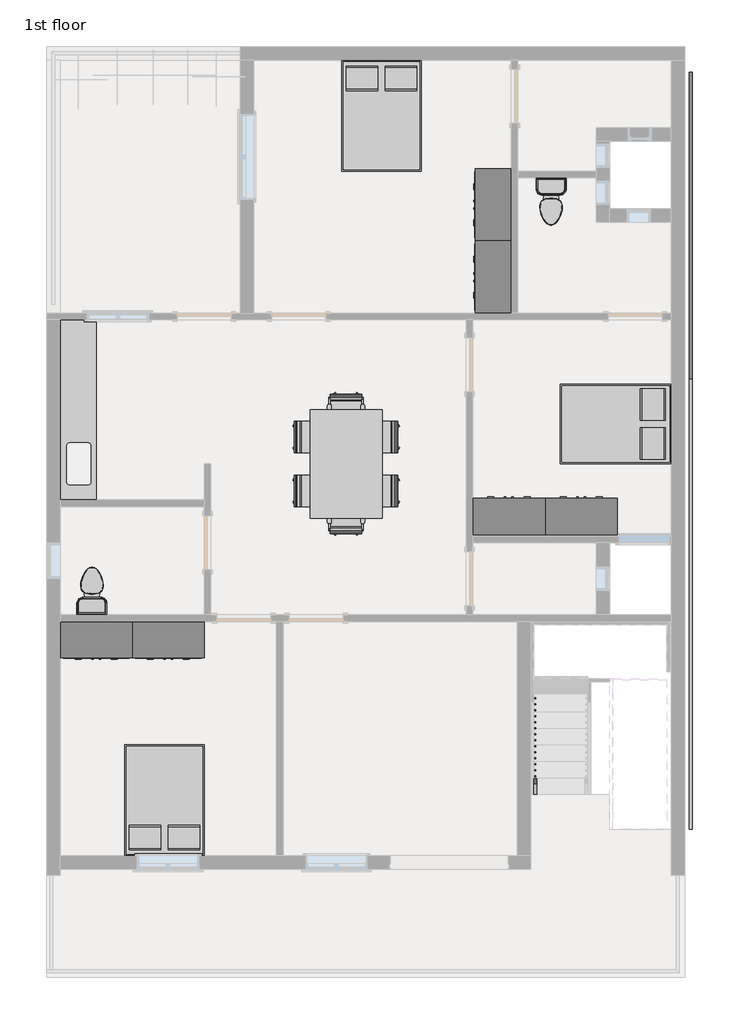
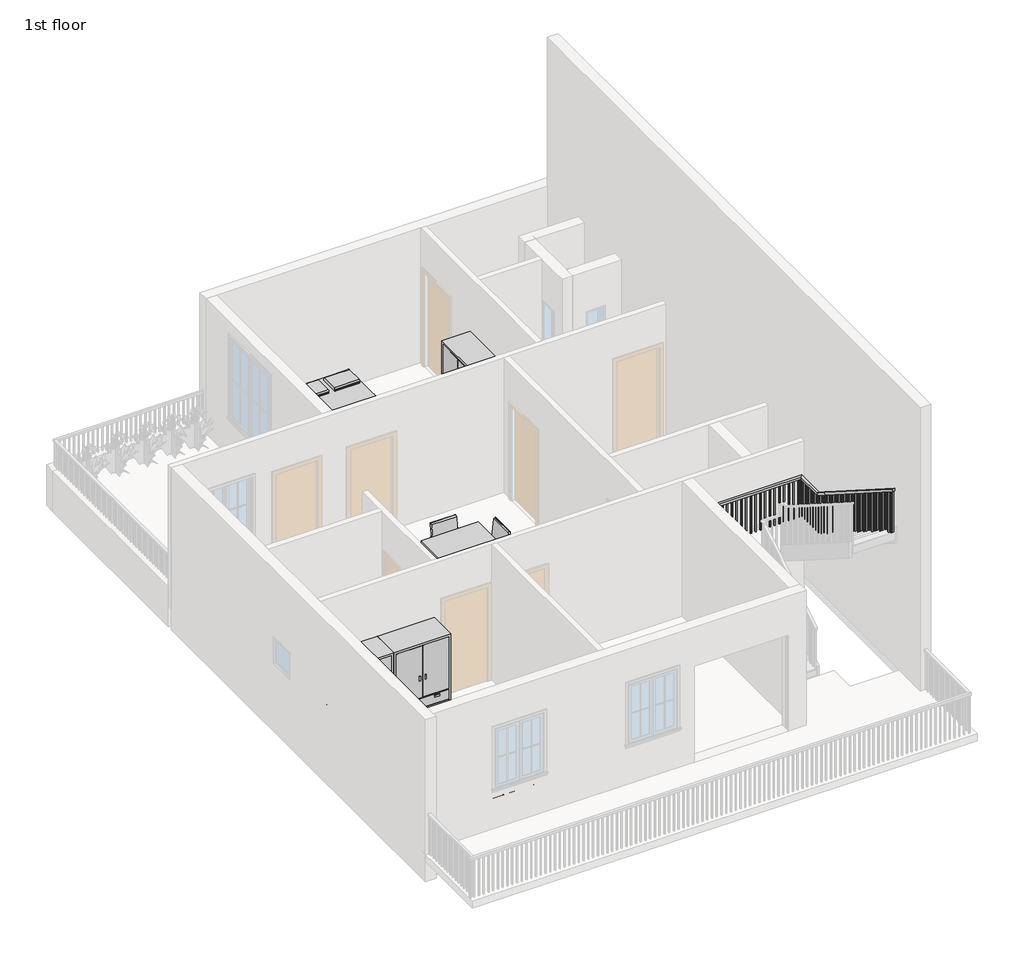
# One storey, part 4 of 5: 18 furniture elements, 2 flow terminals, 1 railing.
"""IFC4 building model written with IfcOpenShell, lengths in millimetres."""

from ifc_helpers import new_model, si_unit, frame, origin, place, context, project, spatial, polyline, outline, extrude, faceted_brep, transform, mapped, element, save
from components import toilet_domestic_3d_toilet_domestic_3d_ba6479b0, toilet_domestic_3d_toilet_domestic_3d_30431060, toilet_domestic_3d_toilet_domestic_3d_9ecb9d01, toilet_domestic_3d_toilet_domestic_3d_e67c3c64, furniture_b58f7881, casework_5_casework_5_bcf4e650, chair_task_chair_task_b7f3823b, chair_task_arms_chair_task_arms_fa5a08ef, furniture_771c7099, furniture_0bcc43ae, furniture_82e269c4

model = new_model("IFC4")

# Units and contexts
model_context = context("Model", 3, world=origin())
ifc_project = project(units=[si_unit("LENGTHUNIT", "METRE", prefix="MILLI")], contexts=[model_context])

# Site, building, storey
site = spatial("IfcSite", under=ifc_project)
building = spatial("IfcBuilding", under=site)
storey = spatial("IfcBuildingStorey", under=building, Name="1st floor", Elevation=3810.0)

# Flow terminals
placement = place(None, origin())
toilet_domestic_3d_toilet_domestic_3d_shape = toilet_domestic_3d_toilet_domestic_3d_ba6479b0(model_context)
toilet_domestic_3d_toilet_domestic_3d_2_shape = toilet_domestic_3d_toilet_domestic_3d_30431060(model_context)
element("IfcFlowTerminal", 1, ObjectType="Toilet-Domestic-3D : Toilet-Domestic-3D", at=placement, inside=storey, context=model_context, shape_type="MappedRepresentation", body=[
    mapped(toilet_domestic_3d_toilet_domestic_3d_shape, transform((424.0501403, 10089.0257925, 3810.0), x_axis=(1.0, 0.0, 0.0), y_axis=(0.0, 1.0, 0.0), z_axis=(0.0, 0.0, 1.0))),
    mapped(toilet_domestic_3d_toilet_domestic_3d_2_shape, transform((424.0501403, 10089.0257925, 3810.0), x_axis=(1.0, 0.0, 0.0), y_axis=(0.0, 1.0, 0.0), z_axis=(0.0, 0.0, 1.0))),
])
toilet_domestic_3d_toilet_domestic_3d_3_shape = toilet_domestic_3d_toilet_domestic_3d_9ecb9d01(model_context)
toilet_domestic_3d_toilet_domestic_3d_4_shape = toilet_domestic_3d_toilet_domestic_3d_e67c3c64(model_context)
element("IfcFlowTerminal", 2, ObjectType="Toilet-Domestic-3D : Toilet-Domestic-3D", at=placement, inside=storey, context=model_context, shape_type="MappedRepresentation", body=[
    mapped(toilet_domestic_3d_toilet_domestic_3d_3_shape, transform((-7342.9058187, 3694.2738062, 3810.0), x_axis=(1.0, 0.0, 0.0), y_axis=(0.0, 1.0, 0.0), z_axis=(0.0, 0.0, 1.0))),
    mapped(toilet_domestic_3d_toilet_domestic_3d_4_shape, transform((-7342.9058187, 3694.2738062, 3810.0), x_axis=(1.0, 0.0, 0.0), y_axis=(0.0, 1.0, 0.0), z_axis=(0.0, 0.0, 1.0))),
])

# Furniture
furniture_shape = furniture_b58f7881(model_context)
element("IfcFurniture", 3, ObjectType="Bed-Box : Double 53\" x 74\"", at=placement, inside=storey, context=model_context, shape_type="MappedRepresentation", body=[
    mapped(furniture_shape, transform((-2785.3023187, 11872.8553007, 3810.0), x_axis=(1.0, 0.0, 0.0), y_axis=(0.0, 1.0, 0.0), z_axis=(0.0, 0.0, 1.0))),
])
element("IfcFurniture", 4, ObjectType="Bed-Box : Double 53\" x 74\"", at=placement, inside=storey, context=model_context, shape_type="MappedRepresentation", body=[
    mapped(furniture_shape, transform((1750.6796485, 6757.8782516, 3810.0), x_axis=(0.0, -1.0, 0.0), y_axis=(1.0, 0.0, 0.0), z_axis=(0.0, 0.0, 1.0))),
])
element("IfcFurniture", 5, ObjectType="Bed-Box : Double 53\" x 74\"", at=placement, inside=storey, context=model_context, shape_type="MappedRepresentation", body=[
    mapped(furniture_shape, transform((-5777.2974007, -178.4037157, 3810.0), x_axis=(-1.0, 0.0, 0.0), y_axis=(0.0, -1.0, 0.0), z_axis=(0.0, 0.0, 1.0))),
])
casework_5_casework_5_shape = casework_5_casework_5_bcf4e650(model_context)
element("IfcFurniture", 6, ObjectType="Casework 5 : Casework 5", at=placement, inside=storey, context=model_context, shape_type="MappedRepresentation", body=[
    mapped(casework_5_casework_5_shape, transform((0.0, 0.0, 0.0), x_axis=(1.0, 0.0, 0.0), y_axis=(0.0, 1.0, 0.0), z_axis=(0.0, 0.0, 1.0))),
])
chair_task_chair_task_shape = chair_task_chair_task_b7f3823b(model_context)
element("IfcFurniture", 7, ObjectType="Chair-Task : Chair-Task", at=placement, inside=storey, context=model_context, shape_type="MappedRepresentation", body=[
    mapped(chair_task_chair_task_shape, transform((-3671.5957614, 6343.8166122, 3810.0), x_axis=(0.0, -1.0, 0.0), y_axis=(1.0, 0.0, 0.0), z_axis=(0.0, 0.0, 1.0))),
])
element("IfcFurniture", 8, ObjectType="Chair-Task : Chair-Task", at=placement, inside=storey, context=model_context, shape_type="MappedRepresentation", body=[
    mapped(chair_task_chair_task_shape, transform((-2414.5039581, 6061.8349729, 3810.0), x_axis=(0.0, 1.0, 0.0), y_axis=(-1.0, 0.0, 0.0), z_axis=(0.0, 0.0, 1.0))),
])
element("IfcFurniture", 9, ObjectType="Chair-Task : Chair-Task", at=placement, inside=storey, context=model_context, shape_type="MappedRepresentation", body=[
    mapped(chair_task_chair_task_shape, transform((-3671.5957614, 5429.4166122, 3810.0), x_axis=(0.0, -1.0, 0.0), y_axis=(1.0, 0.0, 0.0), z_axis=(0.0, 0.0, 1.0))),
])
element("IfcFurniture", 10, ObjectType="Chair-Task : Chair-Task", at=placement, inside=storey, context=model_context, shape_type="MappedRepresentation", body=[
    mapped(chair_task_chair_task_shape, transform((-2414.5039581, 5147.4349729, 3810.0), x_axis=(0.0, 1.0, 0.0), y_axis=(-1.0, 0.0, 0.0), z_axis=(0.0, 0.0, 1.0))),
])
chair_task_arms_chair_task_arms_shape = chair_task_arms_chair_task_arms_fa5a08ef(model_context)
element("IfcFurniture", 11, ObjectType="Chair-Task Arms : Chair-Task Arms", at=placement, inside=storey, context=model_context, shape_type="MappedRepresentation", body=[
    mapped(chair_task_arms_chair_task_arms_shape, transform((-3184.0406794, 4812.2798909, 3810.0), x_axis=(1.0, 0.0, 0.0), y_axis=(0.0, 1.0, 0.0), z_axis=(0.0, 0.0, 1.0))),
])
element("IfcFurniture", 12, ObjectType="Chair-Task Arms : Chair-Task Arms", at=placement, inside=storey, context=model_context, shape_type="MappedRepresentation", body=[
    mapped(chair_task_arms_chair_task_arms_shape, transform((-2902.05904, 6678.9716942, 3810.0), x_axis=(-1.0, 0.0, 0.0), y_axis=(0.0, -1.0, 0.0), z_axis=(0.0, 0.0, 1.0))),
])
furniture_2_shape = furniture_771c7099(model_context)
element("IfcFurniture", 13, ObjectType="Counter Top w Sink Hole : 24\" Depth", at=placement, inside=storey, context=model_context, shape_type="MappedRepresentation", body=[
    mapped(furniture_2_shape, transform((-7907.1498597, 6336.4880876, 3810.0), x_axis=(0.0, 1.0, 0.0), y_axis=(-1.0, 0.0, 0.0), z_axis=(0.0, 0.0, 1.0))),
])
furniture_3_shape = furniture_0bcc43ae(model_context)
element("IfcFurniture", 14, ObjectType="Table-Conference2 w Chairs : 48\" x 144\"", at=placement, inside=storey, context=model_context, shape_type="MappedRepresentation", body=[
    mapped(furniture_3_shape, transform((-3043.0498597, 5745.6257925, 3810.0), x_axis=(0.0, 1.0, 0.0), y_axis=(-1.0, 0.0, 0.0), z_axis=(0.0, 0.0, 1.0))),
])
furniture_4_shape = furniture_82e269c4(model_context)
element("IfcFurniture", 15, ObjectType="Wardrobe : 48\" x 72\" x 24\"", at=placement, inside=storey, context=model_context, shape_type="MappedRepresentation", body=[
    mapped(furniture_4_shape, transform((29.8889499, 8638.7325327, 3810.0), x_axis=(0.0, -1.0, 0.0), y_axis=(1.0, 0.0, 0.0), z_axis=(0.0, 0.0, 1.0))),
])
element("IfcFurniture", 16, ObjectType="Wardrobe : 48\" x 72\" x 24\"", at=placement, inside=storey, context=model_context, shape_type="MappedRepresentation", body=[
    mapped(furniture_4_shape, transform((29.8889499, 9857.9325327, 3810.0), x_axis=(0.0, -1.0, 0.0), y_axis=(1.0, 0.0, 0.0), z_axis=(0.0, 0.0, 1.0))),
])
element("IfcFurniture", 17, ObjectType="Wardrobe : 48\" x 72\" x 24\"", at=placement, inside=storey, context=model_context, shape_type="MappedRepresentation", body=[
    mapped(furniture_4_shape, transform((-556.3431196, 4272.886983, 3810.0), x_axis=(-1.0, 0.0, 0.0), y_axis=(0.0, -1.0, 0.0), z_axis=(0.0, 0.0, 1.0))),
])
element("IfcFurniture", 18, ObjectType="Wardrobe : 48\" x 72\" x 24\"", at=placement, inside=storey, context=model_context, shape_type="MappedRepresentation", body=[
    mapped(furniture_4_shape, transform((662.8568804, 4272.886983, 3810.0), x_axis=(-1.0, 0.0, 0.0), y_axis=(0.0, -1.0, 0.0), z_axis=(0.0, 0.0, 1.0))),
])
element("IfcFurniture", 19, ObjectType="Wardrobe : 48\" x 72\" x 24\"", at=placement, inside=storey, context=model_context, shape_type="MappedRepresentation", body=[
    mapped(furniture_4_shape, transform((-7002.9565999, 3357.5646021, 3810.0), x_axis=(1.0, 0.0, 0.0), y_axis=(0.0, 1.0, 0.0), z_axis=(0.0, 0.0, 1.0))),
])
element("IfcFurniture", 20, ObjectType="Wardrobe : 48\" x 72\" x 24\"", at=placement, inside=storey, context=model_context, shape_type="MappedRepresentation", body=[
    mapped(furniture_4_shape, transform((-5783.7565999, 3357.5646021, 3810.0), x_axis=(1.0, 0.0, 0.0), y_axis=(0.0, 1.0, 0.0), z_axis=(0.0, 0.0, 1.0))),
])

# Railing
element("IfcRailing", 21, ObjectType="Handrail - Rectangular", at=placement, inside=storey, context=model_context, shape_type="SolidModel", body=[
    faceted_brep([(131.9501403, 157.6257925, 4902.2), (131.9501403, 157.6257925, 4841.986276), (182.7501403, 157.6257925, 4841.986276), (182.7501403, 157.6257925, 4902.2), (131.9501403, 2113.4257925, 6146.8), (131.9501403, 2128.2187874, 6096.0), (182.7501403, 2128.2187874, 6096.0), (182.7501403, 2113.4257925, 6146.8), (131.9501403, 3027.8257925, 6146.8), (131.9501403, 3027.8257925, 6096.0), (182.7501403, 2977.0257925, 6096.0), (182.7501403, 2977.0257925, 6146.8), (2379.8501403, 3027.8257925, 6146.8), (2379.8501403, 3027.8257925, 6096.0), (2329.0501403, 2977.0257925, 6096.0), (2329.0501403, 2977.0257925, 6146.8), (2379.8501403, 2392.8257925, 6146.8), (2379.8501403, 2378.0327976, 6096.0), (2329.0501403, 2378.0327976, 6096.0), (2329.0501403, 2392.8257925, 6146.8), (2379.8501403, 2113.4257925, 6324.6), (2379.8501403, 2086.1525175, 6281.7419964), (2329.0501403, 2086.1525175, 6281.7419964), (2329.0501403, 2113.4257925, 6324.6), (2379.8501403, -401.1742075, 7924.8), (2329.0501403, -401.1742075, 7924.8), (2329.0501403, -401.1742075, 7864.586276), (2379.8501403, -401.1742075, 7864.586276)], [[[0, 1, 2, 3]], [[1, 0, 4, 5]], [[2, 1, 5, 6]], [[3, 2, 6, 7]], [[0, 3, 7, 4]], [[5, 4, 8, 9]], [[6, 5, 9, 10]], [[7, 6, 10, 11]], [[4, 7, 11, 8]], [[9, 8, 12, 13]], [[10, 9, 13, 14]], [[11, 10, 14, 15]], [[8, 11, 15, 12]], [[13, 12, 16, 17]], [[14, 13, 17, 18]], [[15, 14, 18, 19]], [[12, 15, 19, 16]], [[17, 16, 20, 21]], [[18, 17, 21, 22]], [[19, 18, 22, 23]], [[16, 19, 23, 20]], [[24, 25, 26, 27]], [[21, 20, 24, 27]], [[22, 21, 27, 26]], [[23, 22, 26, 25]], [[20, 23, 25, 24]]]),
    extrude(outline(polyline([(-315.4492075, 7810.0340032), (-315.4492075, 6832.6), (-334.4992075, 6832.6), (-334.4992075, 7822.1567305), (-315.4492075, 7810.0340032)])), frame((2344.9251403, 0.0, 0.0), z_axis=(1.0, 0.0, 0.0), x_axis=(0.0, 1.0, 0.0)), (0.0, 0.0, 1.0), 19.05),
    extrude(outline(polyline([(-213.8492075, 7745.3794578), (-213.8492075, 6832.6), (-232.8992075, 6832.6), (-232.8992075, 7757.5021851), (-213.8492075, 7745.3794578)])), frame((2344.9251403, 0.0, 0.0), z_axis=(1.0, 0.0, 0.0), x_axis=(0.0, 1.0, 0.0)), (0.0, 0.0, 1.0), 19.05),
    extrude(outline(polyline([(-112.2492075, 7680.7249123), (-112.2492075, 6832.6), (-131.2992075, 6832.6), (-131.2992075, 7692.8476396), (-112.2492075, 7680.7249123)])), frame((2344.9251403, 0.0, 0.0), z_axis=(1.0, 0.0, 0.0), x_axis=(0.0, 1.0, 0.0)), (0.0, 0.0, 1.0), 19.05),
    extrude(outline(polyline([(-10.6492075, 7616.0703669), (-10.6492075, 6654.8), (-29.6992075, 6654.8), (-29.6992075, 7628.1930941), (-10.6492075, 7616.0703669)])), frame((2344.9251403, 0.0, 0.0), z_axis=(1.0, 0.0, 0.0), x_axis=(0.0, 1.0, 0.0)), (0.0, 0.0, 1.0), 19.05),
    extrude(outline(polyline([(90.9507925, 7551.4158214), (90.9507925, 6654.8), (71.9007925, 6654.8), (71.9007925, 7563.5385487), (90.9507925, 7551.4158214)])), frame((2344.9251403, 0.0, 0.0), z_axis=(1.0, 0.0, 0.0), x_axis=(0.0, 1.0, 0.0)), (0.0, 0.0, 1.0), 19.05),
    extrude(outline(polyline([(192.5507925, 7486.761276), (192.5507925, 6477.0), (173.5007925, 6477.0), (173.5007925, 7498.8840032), (192.5507925, 7486.761276)])), frame((2344.9251403, 0.0, 0.0), z_axis=(1.0, 0.0, 0.0), x_axis=(0.0, 1.0, 0.0)), (0.0, 0.0, 1.0), 19.05),
    extrude(outline(polyline([(294.1507925, 7422.1067305), (294.1507925, 6477.0), (275.1007925, 6477.0), (275.1007925, 7434.2294578), (294.1507925, 7422.1067305)])), frame((2344.9251403, 0.0, 0.0), z_axis=(1.0, 0.0, 0.0), x_axis=(0.0, 1.0, 0.0)), (0.0, 0.0, 1.0), 19.05),
    extrude(outline(polyline([(395.7507925, 7357.4521851), (395.7507925, 6477.0), (376.7007925, 6477.0), (376.7007925, 7369.5749123), (395.7507925, 7357.4521851)])), frame((2344.9251403, 0.0, 0.0), z_axis=(1.0, 0.0, 0.0), x_axis=(0.0, 1.0, 0.0)), (0.0, 0.0, 1.0), 19.05),
    extrude(outline(polyline([(497.3507925, 7292.7976396), (497.3507925, 6299.2), (478.3007925, 6299.2), (478.3007925, 7304.9203669), (497.3507925, 7292.7976396)])), frame((2344.9251403, 0.0, 0.0), z_axis=(1.0, 0.0, 0.0), x_axis=(0.0, 1.0, 0.0)), (0.0, 0.0, 1.0), 19.05),
    extrude(outline(polyline([(598.9507925, 7228.1430941), (598.9507925, 6299.2), (579.9007925, 6299.2), (579.9007925, 7240.2658214), (598.9507925, 7228.1430941)])), frame((2344.9251403, 0.0, 0.0), z_axis=(1.0, 0.0, 0.0), x_axis=(0.0, 1.0, 0.0)), (0.0, 0.0, 1.0), 19.05),
    extrude(outline(polyline([(700.5507925, 7163.4885487), (700.5507925, 6299.2), (681.5007925, 6299.2), (681.5007925, 7175.611276), (700.5507925, 7163.4885487)])), frame((2344.9251403, 0.0, 0.0), z_axis=(1.0, 0.0, 0.0), x_axis=(0.0, 1.0, 0.0)), (0.0, 0.0, 1.0), 19.05),
    extrude(outline(polyline([(802.1507925, 7098.8340032), (802.1507925, 6121.4), (783.1007925, 6121.4), (783.1007925, 7110.9567305), (802.1507925, 7098.8340032)])), frame((2344.9251403, 0.0, 0.0), z_axis=(1.0, 0.0, 0.0), x_axis=(0.0, 1.0, 0.0)), (0.0, 0.0, 1.0), 19.05),
    extrude(outline(polyline([(903.7507925, 7034.1794578), (903.7507925, 6121.4), (884.7007925, 6121.4), (884.7007925, 7046.3021851), (903.7507925, 7034.1794578)])), frame((2344.9251403, 0.0, 0.0), z_axis=(1.0, 0.0, 0.0), x_axis=(0.0, 1.0, 0.0)), (0.0, 0.0, 1.0), 19.05),
    extrude(outline(polyline([(1005.3507925, 6969.5249123), (1005.3507925, 6121.4), (986.3007925, 6121.4), (986.3007925, 6981.6476396), (1005.3507925, 6969.5249123)])), frame((2344.9251403, 0.0, 0.0), z_axis=(1.0, 0.0, 0.0), x_axis=(0.0, 1.0, 0.0)), (0.0, 0.0, 1.0), 19.05),
    extrude(outline(polyline([(1106.9507925, 6904.8703669), (1106.9507925, 5943.6), (1087.9007925, 5943.6), (1087.9007925, 6916.9930941), (1106.9507925, 6904.8703669)])), frame((2344.9251403, 0.0, 0.0), z_axis=(1.0, 0.0, 0.0), x_axis=(0.0, 1.0, 0.0)), (0.0, 0.0, 1.0), 19.05),
    extrude(outline(polyline([(1208.5507925, 6840.2158214), (1208.5507925, 5943.6), (1189.5007925, 5943.6), (1189.5007925, 6852.3385487), (1208.5507925, 6840.2158214)])), frame((2344.9251403, 0.0, 0.0), z_axis=(1.0, 0.0, 0.0), x_axis=(0.0, 1.0, 0.0)), (0.0, 0.0, 1.0), 19.05),
    extrude(outline(polyline([(1310.1507925, 6775.561276), (1310.1507925, 5765.8), (1291.1007925, 5765.8), (1291.1007925, 6787.6840032), (1310.1507925, 6775.561276)])), frame((2344.9251403, 0.0, 0.0), z_axis=(1.0, 0.0, 0.0), x_axis=(0.0, 1.0, 0.0)), (0.0, 0.0, 1.0), 19.05),
    extrude(outline(polyline([(1411.7507925, 6710.9067305), (1411.7507925, 5765.8), (1392.7007925, 5765.8), (1392.7007925, 6723.0294578), (1411.7507925, 6710.9067305)])), frame((2344.9251403, 0.0, 0.0), z_axis=(1.0, 0.0, 0.0), x_axis=(0.0, 1.0, 0.0)), (0.0, 0.0, 1.0), 19.05),
    extrude(outline(polyline([(1513.3507925, 6646.2521851), (1513.3507925, 5765.8), (1494.3007925, 5765.8), (1494.3007925, 6658.3749123), (1513.3507925, 6646.2521851)])), frame((2344.9251403, 0.0, 0.0), z_axis=(1.0, 0.0, 0.0), x_axis=(0.0, 1.0, 0.0)), (0.0, 0.0, 1.0), 19.05),
    extrude(outline(polyline([(1614.9507925, 6581.5976396), (1614.9507925, 5588.0), (1595.9007925, 5588.0), (1595.9007925, 6593.7203669), (1614.9507925, 6581.5976396)])), frame((2344.9251403, 0.0, 0.0), z_axis=(1.0, 0.0, 0.0), x_axis=(0.0, 1.0, 0.0)), (0.0, 0.0, 1.0), 19.05),
    extrude(outline(polyline([(1716.5507925, 6516.9430941), (1716.5507925, 5588.0), (1697.5007925, 5588.0), (1697.5007925, 6529.0658214), (1716.5507925, 6516.9430941)])), frame((2344.9251403, 0.0, 0.0), z_axis=(1.0, 0.0, 0.0), x_axis=(0.0, 1.0, 0.0)), (0.0, 0.0, 1.0), 19.05),
    extrude(outline(polyline([(1818.1507925, 6452.2885487), (1818.1507925, 5588.0), (1799.1007925, 5588.0), (1799.1007925, 6464.411276), (1818.1507925, 6452.2885487)])), frame((2344.9251403, 0.0, 0.0), z_axis=(1.0, 0.0, 0.0), x_axis=(0.0, 1.0, 0.0)), (0.0, 0.0, 1.0), 19.05),
    extrude(outline(polyline([(1919.7507925, 6387.6340032), (1919.7507925, 5410.2), (1900.7007925, 5410.2), (1900.7007925, 6399.7567305), (1919.7507925, 6387.6340032)])), frame((2344.9251403, 0.0, 0.0), z_axis=(1.0, 0.0, 0.0), x_axis=(0.0, 1.0, 0.0)), (0.0, 0.0, 1.0), 19.05),
    extrude(outline(polyline([(2021.3507925, 6322.9794578), (2021.3507925, 5410.2), (2002.3007925, 5410.2), (2002.3007925, 6335.1021851), (2021.3507925, 6322.9794578)])), frame((2344.9251403, 0.0, 0.0), z_axis=(1.0, 0.0, 0.0), x_axis=(0.0, 1.0, 0.0)), (0.0, 0.0, 1.0), 19.05),
    extrude(outline(polyline([(2199.1507925, 6209.8340032), (2199.1507925, 5232.4), (2180.1007925, 5232.4), (2180.1007925, 6221.9567305), (2199.1507925, 6209.8340032)])), frame((2344.9251403, 0.0, 0.0), z_axis=(1.0, 0.0, 0.0), x_axis=(0.0, 1.0, 0.0)), (0.0, 0.0, 1.0), 19.05),
    extrude(outline(polyline([(2300.7507925, 6145.1794578), (2300.7507925, 5232.4), (2281.7007925, 5232.4), (2281.7007925, 6157.3021851), (2300.7507925, 6145.1794578)])), frame((2344.9251403, 0.0, 0.0), z_axis=(1.0, 0.0, 0.0), x_axis=(0.0, 1.0, 0.0)), (0.0, 0.0, 1.0), 19.05),
    extrude(outline(polyline([(2363.9751403, 2402.3507925), (2363.9751403, 2383.3007925), (2344.9251403, 2383.3007925), (2344.9251403, 2402.3507925), (2363.9751403, 2402.3507925)])), frame((0.0, 0.0, 5232.4), z_axis=(0.0, 0.0, 1.0), x_axis=(1.0, 0.0, 0.0)), (0.0, 0.0, 1.0), 863.6),
    extrude(outline(polyline([(2363.9751403, 2503.9507925), (2363.9751403, 2484.9007925), (2344.9251403, 2484.9007925), (2344.9251403, 2503.9507925), (2363.9751403, 2503.9507925)])), frame((0.0, 0.0, 5232.4), z_axis=(0.0, 0.0, 1.0), x_axis=(1.0, 0.0, 0.0)), (0.0, 0.0, 1.0), 863.6),
    extrude(outline(polyline([(2363.9751403, 2605.5507925), (2363.9751403, 2586.5007925), (2344.9251403, 2586.5007925), (2344.9251403, 2605.5507925), (2363.9751403, 2605.5507925)])), frame((0.0, 0.0, 5232.4), z_axis=(0.0, 0.0, 1.0), x_axis=(1.0, 0.0, 0.0)), (0.0, 0.0, 1.0), 863.6),
    extrude(outline(polyline([(2363.9751403, 2707.1507925), (2363.9751403, 2688.1007925), (2344.9251403, 2688.1007925), (2344.9251403, 2707.1507925), (2363.9751403, 2707.1507925)])), frame((0.0, 0.0, 5232.4), z_axis=(0.0, 0.0, 1.0), x_axis=(1.0, 0.0, 0.0)), (0.0, 0.0, 1.0), 863.6),
    extrude(outline(polyline([(2363.9751403, 2808.7507925), (2363.9751403, 2789.7007925), (2344.9251403, 2789.7007925), (2344.9251403, 2808.7507925), (2363.9751403, 2808.7507925)])), frame((0.0, 0.0, 5232.4), z_axis=(0.0, 0.0, 1.0), x_axis=(1.0, 0.0, 0.0)), (0.0, 0.0, 1.0), 863.6),
    extrude(outline(polyline([(2363.9751403, 2910.3507925), (2363.9751403, 2891.3007925), (2344.9251403, 2891.3007925), (2344.9251403, 2910.3507925), (2363.9751403, 2910.3507925)])), frame((0.0, 0.0, 5232.4), z_axis=(0.0, 0.0, 1.0), x_axis=(1.0, 0.0, 0.0)), (0.0, 0.0, 1.0), 863.6),
    extrude(outline(polyline([(2281.4251403, 3011.9507925), (2300.4751403, 3011.9507925), (2300.4751403, 2992.9007925), (2281.4251403, 2992.9007925), (2281.4251403, 3011.9507925)])), frame((0.0, 0.0, 5232.4), z_axis=(0.0, 0.0, 1.0), x_axis=(1.0, 0.0, 0.0)), (0.0, 0.0, 1.0), 863.6),
    extrude(outline(polyline([(2179.8251403, 3011.9507925), (2198.8751403, 3011.9507925), (2198.8751403, 2992.9007925), (2179.8251403, 2992.9007925), (2179.8251403, 3011.9507925)])), frame((0.0, 0.0, 5232.4), z_axis=(0.0, 0.0, 1.0), x_axis=(1.0, 0.0, 0.0)), (0.0, 0.0, 1.0), 863.6),
    extrude(outline(polyline([(2078.2251403, 3011.9507925), (2097.2751403, 3011.9507925), (2097.2751403, 2992.9007925), (2078.2251403, 2992.9007925), (2078.2251403, 3011.9507925)])), frame((0.0, 0.0, 5232.4), z_axis=(0.0, 0.0, 1.0), x_axis=(1.0, 0.0, 0.0)), (0.0, 0.0, 1.0), 863.6),
    extrude(outline(polyline([(1976.6251403, 3011.9507925), (1995.6751403, 3011.9507925), (1995.6751403, 2992.9007925), (1976.6251403, 2992.9007925), (1976.6251403, 3011.9507925)])), frame((0.0, 0.0, 5232.4), z_axis=(0.0, 0.0, 1.0), x_axis=(1.0, 0.0, 0.0)), (0.0, 0.0, 1.0), 863.6),
    extrude(outline(polyline([(1875.0251403, 3011.9507925), (1894.0751403, 3011.9507925), (1894.0751403, 2992.9007925), (1875.0251403, 2992.9007925), (1875.0251403, 3011.9507925)])), frame((0.0, 0.0, 5232.4), z_axis=(0.0, 0.0, 1.0), x_axis=(1.0, 0.0, 0.0)), (0.0, 0.0, 1.0), 863.6),
    extrude(outline(polyline([(1773.4251403, 3011.9507925), (1792.4751403, 3011.9507925), (1792.4751403, 2992.9007925), (1773.4251403, 2992.9007925), (1773.4251403, 3011.9507925)])), frame((0.0, 0.0, 5232.4), z_axis=(0.0, 0.0, 1.0), x_axis=(1.0, 0.0, 0.0)), (0.0, 0.0, 1.0), 863.6),
    extrude(outline(polyline([(1671.8251403, 3011.9507925), (1690.8751403, 3011.9507925), (1690.8751403, 2992.9007925), (1671.8251403, 2992.9007925), (1671.8251403, 3011.9507925)])), frame((0.0, 0.0, 5232.4), z_axis=(0.0, 0.0, 1.0), x_axis=(1.0, 0.0, 0.0)), (0.0, 0.0, 1.0), 863.6),
    extrude(outline(polyline([(1570.2251403, 3011.9507925), (1589.2751403, 3011.9507925), (1589.2751403, 2992.9007925), (1570.2251403, 2992.9007925), (1570.2251403, 3011.9507925)])), frame((0.0, 0.0, 5232.4), z_axis=(0.0, 0.0, 1.0), x_axis=(1.0, 0.0, 0.0)), (0.0, 0.0, 1.0), 863.6),
    extrude(outline(polyline([(1468.6251403, 3011.9507925), (1487.6751403, 3011.9507925), (1487.6751403, 2992.9007925), (1468.6251403, 2992.9007925), (1468.6251403, 3011.9507925)])), frame((0.0, 0.0, 5232.4), z_axis=(0.0, 0.0, 1.0), x_axis=(1.0, 0.0, 0.0)), (0.0, 0.0, 1.0), 863.6),
    extrude(outline(polyline([(1367.0251403, 3011.9507925), (1386.0751403, 3011.9507925), (1386.0751403, 2992.9007925), (1367.0251403, 2992.9007925), (1367.0251403, 3011.9507925)])), frame((0.0, 0.0, 5232.4), z_axis=(0.0, 0.0, 1.0), x_axis=(1.0, 0.0, 0.0)), (0.0, 0.0, 1.0), 863.6),
    extrude(outline(polyline([(1265.4251403, 3011.9507925), (1284.4751403, 3011.9507925), (1284.4751403, 2992.9007925), (1265.4251403, 2992.9007925), (1265.4251403, 3011.9507925)])), frame((0.0, 0.0, 5232.4), z_axis=(0.0, 0.0, 1.0), x_axis=(1.0, 0.0, 0.0)), (0.0, 0.0, 1.0), 863.6),
    extrude(outline(polyline([(1163.8251403, 3011.9507925), (1182.8751403, 3011.9507925), (1182.8751403, 2992.9007925), (1163.8251403, 2992.9007925), (1163.8251403, 3011.9507925)])), frame((0.0, 0.0, 5232.4), z_axis=(0.0, 0.0, 1.0), x_axis=(1.0, 0.0, 0.0)), (0.0, 0.0, 1.0), 863.6),
    extrude(outline(polyline([(1062.2251403, 3011.9507925), (1081.2751403, 3011.9507925), (1081.2751403, 2992.9007925), (1062.2251403, 2992.9007925), (1062.2251403, 3011.9507925)])), frame((0.0, 0.0, 5232.4), z_axis=(0.0, 0.0, 1.0), x_axis=(1.0, 0.0, 0.0)), (0.0, 0.0, 1.0), 863.6),
    extrude(outline(polyline([(960.6251403, 3011.9507925), (979.6751403, 3011.9507925), (979.6751403, 2992.9007925), (960.6251403, 2992.9007925), (960.6251403, 3011.9507925)])), frame((0.0, 0.0, 5232.4), z_axis=(0.0, 0.0, 1.0), x_axis=(1.0, 0.0, 0.0)), (0.0, 0.0, 1.0), 863.6),
    extrude(outline(polyline([(859.0251403, 3011.9507925), (878.0751403, 3011.9507925), (878.0751403, 2992.9007925), (859.0251403, 2992.9007925), (859.0251403, 3011.9507925)])), frame((0.0, 0.0, 5232.4), z_axis=(0.0, 0.0, 1.0), x_axis=(1.0, 0.0, 0.0)), (0.0, 0.0, 1.0), 863.6),
    extrude(outline(polyline([(757.4251403, 3011.9507925), (776.4751403, 3011.9507925), (776.4751403, 2992.9007925), (757.4251403, 2992.9007925), (757.4251403, 3011.9507925)])), frame((0.0, 0.0, 5232.4), z_axis=(0.0, 0.0, 1.0), x_axis=(1.0, 0.0, 0.0)), (0.0, 0.0, 1.0), 863.6),
    extrude(outline(polyline([(655.8251403, 3011.9507925), (674.8751403, 3011.9507925), (674.8751403, 2992.9007925), (655.8251403, 2992.9007925), (655.8251403, 3011.9507925)])), frame((0.0, 0.0, 5232.4), z_axis=(0.0, 0.0, 1.0), x_axis=(1.0, 0.0, 0.0)), (0.0, 0.0, 1.0), 863.6),
    extrude(outline(polyline([(554.2251403, 3011.9507925), (573.2751403, 3011.9507925), (573.2751403, 2992.9007925), (554.2251403, 2992.9007925), (554.2251403, 3011.9507925)])), frame((0.0, 0.0, 5232.4), z_axis=(0.0, 0.0, 1.0), x_axis=(1.0, 0.0, 0.0)), (0.0, 0.0, 1.0), 863.6),
    extrude(outline(polyline([(452.6251403, 3011.9507925), (471.6751403, 3011.9507925), (471.6751403, 2992.9007925), (452.6251403, 2992.9007925), (452.6251403, 3011.9507925)])), frame((0.0, 0.0, 5232.4), z_axis=(0.0, 0.0, 1.0), x_axis=(1.0, 0.0, 0.0)), (0.0, 0.0, 1.0), 863.6),
    extrude(outline(polyline([(351.0251403, 3011.9507925), (370.0751403, 3011.9507925), (370.0751403, 2992.9007925), (351.0251403, 2992.9007925), (351.0251403, 3011.9507925)])), frame((0.0, 0.0, 5232.4), z_axis=(0.0, 0.0, 1.0), x_axis=(1.0, 0.0, 0.0)), (0.0, 0.0, 1.0), 863.6),
    extrude(outline(polyline([(249.4251403, 3011.9507925), (268.4751403, 3011.9507925), (268.4751403, 2992.9007925), (249.4251403, 2992.9007925), (249.4251403, 3011.9507925)])), frame((0.0, 0.0, 5232.4), z_axis=(0.0, 0.0, 1.0), x_axis=(1.0, 0.0, 0.0)), (0.0, 0.0, 1.0), 863.6),
    extrude(outline(polyline([(147.8251403, 2916.7007925), (147.8251403, 2935.7507925), (166.8751403, 2935.7507925), (166.8751403, 2916.7007925), (147.8251403, 2916.7007925)])), frame((0.0, 0.0, 5232.4), z_axis=(0.0, 0.0, 1.0), x_axis=(1.0, 0.0, 0.0)), (0.0, 0.0, 1.0), 863.6),
    extrude(outline(polyline([(147.8251403, 2815.1007925), (147.8251403, 2834.1507925), (166.8751403, 2834.1507925), (166.8751403, 2815.1007925), (147.8251403, 2815.1007925)])), frame((0.0, 0.0, 5232.4), z_axis=(0.0, 0.0, 1.0), x_axis=(1.0, 0.0, 0.0)), (0.0, 0.0, 1.0), 863.6),
    extrude(outline(polyline([(147.8251403, 2713.5007925), (147.8251403, 2732.5507925), (166.8751403, 2732.5507925), (166.8751403, 2713.5007925), (147.8251403, 2713.5007925)])), frame((0.0, 0.0, 5232.4), z_axis=(0.0, 0.0, 1.0), x_axis=(1.0, 0.0, 0.0)), (0.0, 0.0, 1.0), 863.6),
    extrude(outline(polyline([(147.8251403, 2611.9007925), (147.8251403, 2630.9507925), (166.8751403, 2630.9507925), (166.8751403, 2611.9007925), (147.8251403, 2611.9007925)])), frame((0.0, 0.0, 5232.4), z_axis=(0.0, 0.0, 1.0), x_axis=(1.0, 0.0, 0.0)), (0.0, 0.0, 1.0), 863.6),
    extrude(outline(polyline([(147.8251403, 2510.3007925), (147.8251403, 2529.3507925), (166.8751403, 2529.3507925), (166.8751403, 2510.3007925), (147.8251403, 2510.3007925)])), frame((0.0, 0.0, 5232.4), z_axis=(0.0, 0.0, 1.0), x_axis=(1.0, 0.0, 0.0)), (0.0, 0.0, 1.0), 863.6),
    extrude(outline(polyline([(147.8251403, 2408.7007925), (147.8251403, 2427.7507925), (166.8751403, 2427.7507925), (166.8751403, 2408.7007925), (147.8251403, 2408.7007925)])), frame((0.0, 0.0, 5232.4), z_axis=(0.0, 0.0, 1.0), x_axis=(1.0, 0.0, 0.0)), (0.0, 0.0, 1.0), 863.6),
    extrude(outline(polyline([(147.8251403, 2307.1007925), (147.8251403, 2326.1507925), (166.8751403, 2326.1507925), (166.8751403, 2307.1007925), (147.8251403, 2307.1007925)])), frame((0.0, 0.0, 5232.4), z_axis=(0.0, 0.0, 1.0), x_axis=(1.0, 0.0, 0.0)), (0.0, 0.0, 1.0), 863.6),
    extrude(outline(polyline([(147.8251403, 2205.5007925), (147.8251403, 2224.5507925), (166.8751403, 2224.5507925), (166.8751403, 2205.5007925), (147.8251403, 2205.5007925)])), frame((0.0, 0.0, 5232.4), z_axis=(0.0, 0.0, 1.0), x_axis=(1.0, 0.0, 0.0)), (0.0, 0.0, 1.0), 863.6),
    extrude(outline(polyline([(2097.5507925, 6076.4840032), (2097.5507925, 5054.6), (2078.5007925, 5054.6), (2078.5007925, 6064.361276), (2097.5507925, 6076.4840032)])), frame((147.8251403, 0.0, 0.0), z_axis=(1.0, 0.0, 0.0), x_axis=(0.0, 1.0, 0.0)), (0.0, 0.0, 1.0), 19.05),
    extrude(outline(polyline([(1995.9507925, 6011.8294578), (1995.9507925, 5054.6), (1976.9007925, 5054.6), (1976.9007925, 5999.7067305), (1995.9507925, 6011.8294578)])), frame((147.8251403, 0.0, 0.0), z_axis=(1.0, 0.0, 0.0), x_axis=(0.0, 1.0, 0.0)), (0.0, 0.0, 1.0), 19.05),
    extrude(outline(polyline([(1894.3507925, 5947.1749123), (1894.3507925, 5054.6), (1875.3007925, 5054.6), (1875.3007925, 5935.0521851), (1894.3507925, 5947.1749123)])), frame((147.8251403, 0.0, 0.0), z_axis=(1.0, 0.0, 0.0), x_axis=(0.0, 1.0, 0.0)), (0.0, 0.0, 1.0), 19.05),
    extrude(outline(polyline([(1792.7507925, 5882.5203669), (1792.7507925, 4876.8), (1773.7007925, 4876.8), (1773.7007925, 5870.3976396), (1792.7507925, 5882.5203669)])), frame((147.8251403, 0.0, 0.0), z_axis=(1.0, 0.0, 0.0), x_axis=(0.0, 1.0, 0.0)), (0.0, 0.0, 1.0), 19.05),
    extrude(outline(polyline([(1691.1507925, 5817.8658214), (1691.1507925, 4876.8), (1672.1007925, 4876.8), (1672.1007925, 5805.7430941), (1691.1507925, 5817.8658214)])), frame((147.8251403, 0.0, 0.0), z_axis=(1.0, 0.0, 0.0), x_axis=(0.0, 1.0, 0.0)), (0.0, 0.0, 1.0), 19.05),
    extrude(outline(polyline([(1589.5507925, 5753.211276), (1589.5507925, 4876.8), (1570.5007925, 4876.8), (1570.5007925, 5741.0885487), (1589.5507925, 5753.211276)])), frame((147.8251403, 0.0, 0.0), z_axis=(1.0, 0.0, 0.0), x_axis=(0.0, 1.0, 0.0)), (0.0, 0.0, 1.0), 19.05),
    extrude(outline(polyline([(1487.9507925, 5688.5567305), (1487.9507925, 4699.0), (1468.9007925, 4699.0), (1468.9007925, 5676.4340032), (1487.9507925, 5688.5567305)])), frame((147.8251403, 0.0, 0.0), z_axis=(1.0, 0.0, 0.0), x_axis=(0.0, 1.0, 0.0)), (0.0, 0.0, 1.0), 19.05),
    extrude(outline(polyline([(1386.3507925, 5623.9021851), (1386.3507925, 4699.0), (1367.3007925, 4699.0), (1367.3007925, 5611.7794578), (1386.3507925, 5623.9021851)])), frame((147.8251403, 0.0, 0.0), z_axis=(1.0, 0.0, 0.0), x_axis=(0.0, 1.0, 0.0)), (0.0, 0.0, 1.0), 19.05),
    extrude(outline(polyline([(1284.7507925, 5559.2476396), (1284.7507925, 4699.0), (1265.7007925, 4699.0), (1265.7007925, 5547.1249123), (1284.7507925, 5559.2476396)])), frame((147.8251403, 0.0, 0.0), z_axis=(1.0, 0.0, 0.0), x_axis=(0.0, 1.0, 0.0)), (0.0, 0.0, 1.0), 19.05),
    extrude(outline(polyline([(1183.1507925, 5494.5930941), (1183.1507925, 4521.2), (1164.1007925, 4521.2), (1164.1007925, 5482.4703669), (1183.1507925, 5494.5930941)])), frame((147.8251403, 0.0, 0.0), z_axis=(1.0, 0.0, 0.0), x_axis=(0.0, 1.0, 0.0)), (0.0, 0.0, 1.0), 19.05),
    extrude(outline(polyline([(1081.5507925, 5429.9385487), (1081.5507925, 4521.2), (1062.5007925, 4521.2), (1062.5007925, 5417.8158214), (1081.5507925, 5429.9385487)])), frame((147.8251403, 0.0, 0.0), z_axis=(1.0, 0.0, 0.0), x_axis=(0.0, 1.0, 0.0)), (0.0, 0.0, 1.0), 19.05),
    extrude(outline(polyline([(979.9507925, 5365.2840032), (979.9507925, 4343.4), (960.9007925, 4343.4), (960.9007925, 5353.161276), (979.9507925, 5365.2840032)])), frame((147.8251403, 0.0, 0.0), z_axis=(1.0, 0.0, 0.0), x_axis=(0.0, 1.0, 0.0)), (0.0, 0.0, 1.0), 19.05),
    extrude(outline(polyline([(878.3507925, 5300.6294578), (878.3507925, 4343.4), (859.3007925, 4343.4), (859.3007925, 5288.5067305), (878.3507925, 5300.6294578)])), frame((147.8251403, 0.0, 0.0), z_axis=(1.0, 0.0, 0.0), x_axis=(0.0, 1.0, 0.0)), (0.0, 0.0, 1.0), 19.05),
    extrude(outline(polyline([(776.7507925, 5235.9749123), (776.7507925, 4343.4), (757.7007925, 4343.4), (757.7007925, 5223.8521851), (776.7507925, 5235.9749123)])), frame((147.8251403, 0.0, 0.0), z_axis=(1.0, 0.0, 0.0), x_axis=(0.0, 1.0, 0.0)), (0.0, 0.0, 1.0), 19.05),
    extrude(outline(polyline([(675.1507925, 5171.3203669), (675.1507925, 4165.6), (656.1007925, 4165.6), (656.1007925, 5159.1976396), (675.1507925, 5171.3203669)])), frame((147.8251403, 0.0, 0.0), z_axis=(1.0, 0.0, 0.0), x_axis=(0.0, 1.0, 0.0)), (0.0, 0.0, 1.0), 19.05),
    extrude(outline(polyline([(573.5507925, 5106.6658214), (573.5507925, 4165.6), (554.5007925, 4165.6), (554.5007925, 5094.5430941), (573.5507925, 5106.6658214)])), frame((147.8251403, 0.0, 0.0), z_axis=(1.0, 0.0, 0.0), x_axis=(0.0, 1.0, 0.0)), (0.0, 0.0, 1.0), 19.05),
    extrude(outline(polyline([(471.9507925, 5042.011276), (471.9507925, 4165.6), (452.9007925, 4165.6), (452.9007925, 5029.8885487), (471.9507925, 5042.011276)])), frame((147.8251403, 0.0, 0.0), z_axis=(1.0, 0.0, 0.0), x_axis=(0.0, 1.0, 0.0)), (0.0, 0.0, 1.0), 19.05),
    extrude(outline(polyline([(370.3507925, 4977.3567305), (370.3507925, 3987.8), (351.3007925, 3987.8), (351.3007925, 4965.2340032), (370.3507925, 4977.3567305)])), frame((147.8251403, 0.0, 0.0), z_axis=(1.0, 0.0, 0.0), x_axis=(0.0, 1.0, 0.0)), (0.0, 0.0, 1.0), 19.05),
    extrude(outline(polyline([(268.7507925, 4912.7021851), (268.7507925, 3987.8), (249.7007925, 3987.8), (249.7007925, 4900.5794578), (268.7507925, 4912.7021851)])), frame((147.8251403, 0.0, 0.0), z_axis=(1.0, 0.0, 0.0), x_axis=(0.0, 1.0, 0.0)), (0.0, 0.0, 1.0), 19.05),
    extrude(outline(polyline([(2122.9507925, 6258.3249123), (2122.9507925, 5232.4), (2103.9007925, 5232.4), (2103.9007925, 6270.4476396), (2122.9507925, 6258.3249123)])), frame((2344.9251403, 0.0, 0.0), z_axis=(1.0, 0.0, 0.0), x_axis=(0.0, 1.0, 0.0)), (0.0, 0.0, 1.0), 19.05),
    extrude(outline(polyline([(2344.9251403, 3011.9507925), (2363.9751403, 3011.9507925), (2363.9751403, 2992.9007925), (2344.9251403, 2992.9007925), (2344.9251403, 3011.9507925)])), frame((0.0, 0.0, 5232.4), z_axis=(0.0, 0.0, 1.0), x_axis=(1.0, 0.0, 0.0)), (0.0, 0.0, 1.0), 863.6),
    extrude(outline(polyline([(147.8251403, 2992.9007925), (147.8251403, 3011.9507925), (166.8751403, 3011.9507925), (166.8751403, 2992.9007925), (147.8251403, 2992.9007925)])), frame((0.0, 0.0, 5232.4), z_axis=(0.0, 0.0, 1.0), x_axis=(1.0, 0.0, 0.0)), (0.0, 0.0, 1.0), 863.6),
    extrude(outline(polyline([(2122.9507925, 6092.6476396), (2122.9507925, 5232.4), (2103.9007925, 5232.4), (2103.9007925, 6080.5249123), (2122.9507925, 6092.6476396)])), frame((147.8251403, 0.0, 0.0), z_axis=(1.0, 0.0, 0.0), x_axis=(0.0, 1.0, 0.0)), (0.0, 0.0, 1.0), 19.05),
    extrude(outline(polyline([(-382.1242075, 7852.4635487), (-382.1242075, 6832.6), (-401.1742075, 6832.6), (-401.1742075, 7864.586276), (-382.1242075, 7852.4635487)])), frame((2344.9251403, 0.0, 0.0), z_axis=(1.0, 0.0, 0.0), x_axis=(0.0, 1.0, 0.0)), (0.0, 0.0, 1.0), 19.05),
    extrude(outline(polyline([(176.6757925, 4854.1090032), (176.6757925, 3987.8), (157.6257925, 3987.8), (157.6257925, 4841.986276), (176.6757925, 4854.1090032)])), frame((147.8251403, 0.0, 0.0), z_axis=(1.0, 0.0, 0.0), x_axis=(0.0, 1.0, 0.0)), (0.0, 0.0, 1.0), 19.05),
])

save(model, "model.ifc")

# Revit data of these elements
# Type "Toilet-Domestic-3D : Toilet-Domestic-3D"
#   Assembly Code = "D2010110"
#   Toilet - Bowl/Basin Material = Porcelain, Linen
#   Toilet - Seat Material = Laminate, Linen, Matte
#   Default Elevation = 0
# Type "Bed-Box : Double 53\" x 74\""
#   Assembly Code = "E2020200"
#   Length = 6' - 2"
#   Width = 4' - 5"
#   Frame Material = Birch
#   Mattress Material = Linen, White
#   Default Elevation = 0
# Type "Chair-Task : Chair-Task"
#   Assembly Code = "E2020200"
#   Base Material = Plastic - Black
#   Caster Material = Plastic - Black
#   Seat/Back Material = Textile - Slate Blue
#   Default Elevation = 0
# Type "Chair-Task Arms : Chair-Task Arms"
#   Assembly Code = "E2020200"
#   Base Material = Plastic - Black
#   Caster Material = Plastic - Black
#   Seat/Back Material = Textile - Slate Blue
#   Default Elevation = 0
# Type "Counter Top w Sink Hole : 24\" Depth"
#   Assembly Code = "C1030400"
#   Counter Thickness = 0' - 1 1/2"
#   Depth = 2' - 1"
#   Height = 3' - 0"
#   Length [instance default] = 8' - 0"
#   Sink Location [instance default] = 2' - 0"
#   Sink Location To Wall [instance default] = 0' - 6"
#   Sink Opening Depth [instance default] = 1' - 3"
#   Sink Opening Width [instance default] = 2' - 3"
#   Counter Top Material = none
#   Default Elevation = 0
# Type "Table-Conference2 w Chairs : 48\" x 144\""
#   Assembly Code = "E2020200"
#   Description = "Seating 12-14"
#   Height = 2' - 6"
#   Length = 6' - 0"
#   Width = 4' - 0"
#   Number Of Chairs One Side = 2
#   Number Of Chairs = 6
#   Material = Wood - Cherry
#   Default Elevation = 0
# Type "Wardrobe : 48\" x 72\" x 24\""
#   Assembly Code = "E2020200"
#   Depth = 2' - 0"
#   Height = 6' - 0"
#   Width = 4' - 0"
#   Material = Wood - Mahogany
#   Default Elevation = 0
# Type "Handrail - Rectangular"
#   Assembly Code = "C2010400"
#   built-in parameter 1008612 = 0.0416667 (stored number, unit not read)
#   built-in parameter 1008611 = 0.0416667 (stored number, unit not read)
#   built-in parameter 1008609 = 0.333333 (stored number, unit not read)
#   built-in parameter 1008604 = 0.166667 (stored number, unit not read)
#   built-in parameter 1008603 = 0.166667 (stored number, unit not read)
#   Railing Height = 3' - 0"
#   built-in parameter 1008630 = 2
#   built-in parameter 1008610 = 2
#   built-in parameter 1008618 = Baluster - Square : 3/4"
# Element 1 (IfcFlowTerminal, "Toilet-Domestic-3D : Toilet-Domestic-3D")
#   Mark = "8"
#   Phase Created = New Construction
#   Materials on its faces: "Porcelain, Linen", "Laminate, Linen, Matte"
# Element 2 (IfcFlowTerminal, "Toilet-Domestic-3D : Toilet-Domestic-3D")
#   Mark = "7"
#   Phase Created = New Construction
#   Materials on its faces: "Porcelain, Linen", "Laminate, Linen, Matte"
# Elements 3, 4, 5 (IfcFurniture, "Bed-Box : Double 53\" x 74\"")
#   Phase Created = New Construction
#   Materials on its faces: "Birch", "Linen, White"
# Element 6 (IfcFurniture, "Casework 5 : Casework 5")
#   Phase Created = New Construction
#   Materials on its faces: "Linen, White"
# Elements 7, 8, 9, 10 (IfcFurniture, "Chair-Task : Chair-Task")
#   Phase Created = New Construction
#   Materials on its faces: "Plastic - Black", "Textile - Slate Blue"
# Elements 11, 12 (IfcFurniture, "Chair-Task Arms : Chair-Task Arms")
#   Phase Created = New Construction
#   Materials on its faces: "Plastic - Black", "Textile - Slate Blue"
# Element 13 (IfcFurniture, "Counter Top w Sink Hole : 24\" Depth")
#   Sink Opening Width = 2' - 3"
#   Sink Opening Depth = 1' - 3"
#   Sink Location To Wall = 0' - 6"
#   Sink Location = 2' - 0"
#   Length = 10' - 0"
#   Phase Created = New Construction
#   Materials on its faces: "Counter Top"
# Element 14 (IfcFurniture, "Table-Conference2 w Chairs : 48\" x 144\"")
#   Phase Created = New Construction
#   Materials on its faces: "Wood - Cherry"
# Elements 15, 16, 17, 18, 19, 20 (IfcFurniture, "Wardrobe : 48\" x 72\" x 24\"")
#   Phase Created = New Construction
#   Materials on its faces: "Wood - Mahogany"
# Element 21 (IfcRailing, "Handrail - Rectangular")
#   Phase Created = New Construction
# Materials
#   "Porcelain, Linen": class "Ceramic", colour RGB 249 239 230, transparency 0, Description = "Porcelain, linen", Cost = 0
#   "Laminate, Linen, Matte": class "Plastic", colour RGB 249 239 230, transparency 0, Description = "Plastic Laminate - Linen, Matte", Cost = 0
#   "Birch": class "Wood", colour RGB 224 178 126, transparency 0, Description = "Betula Alleghaniensis", Cost = 0
#   "Linen, White": class "Textile", colour RGB 247 247 239, transparency 0, Description = "Linen, white", Cost = 0
#   "Plastic - Black": colour RGB 0 0 0, transparency 0.7
#   "Textile - Slate Blue": colour RGB 98 102 118, transparency 0
#   "Wood - Cherry": colour RGB 151 75 0, transparency 0
#   "Wood - Mahogany": colour RGB 138 86 45, transparency 0
#   "Counter Top": class "Wood", colour RGB 226 177 128, transparency 0
